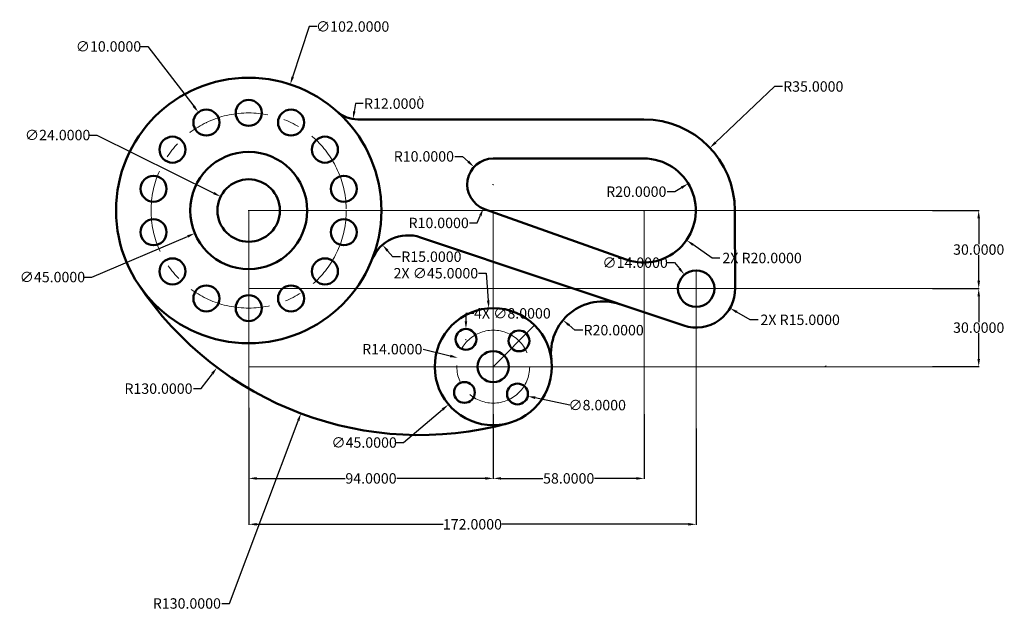
# Model space of a CAD drawing. Units: inches. Extents: x 647 to 1025, y 654 to 881.
import ezdxf

# ---------------------------------------------------------------- set-up
doc = ezdxf.new("R2010")
doc.units = ezdxf.units.IN
doc.header["$MEASUREMENT"] = 0
doc.linetypes.add('CENTER', pattern=[50.8, 31.75, -6.35, 6.35, -6.35])
for name, color, linetype, lineweight in [('M-CNTR', 240, 'CENTER', 18), ('M-CONS', 240, 'Continuous', 13), ('M-DIMS', 2, 'Continuous', 25), ('M-OUTL', 7, 'Continuous', 50)]:
    doc.layers.add(name, color=color, linetype=linetype, lineweight=lineweight)
doc.styles.get("Standard").update_dxf_attribs({"font": 'arial.ttf'})
doc.dimstyles.get("Standard").update_dxf_attribs({"dimtxt": 4, "dimasz": 3, "dimexe": 0.18, "dimexo": 0.0625, "dimgap": 0.09, "dimtad": 0, "dimtih": 1, "dimtoh": 1, "dimdec": 4, "dimzin": 0, "dimdsep": 46, "dimtxsty": 'Standard', "dimcen": 0.09, "dimadec": 0, "dimazin": 0, "dimtfac": 1, "dimtdec": 4, "dimtofl": 0, "dimtmove": 0, "dimatfit": 3, "dimfxl": 1, "dimtolj": 1, "dimtzin": 0, "dimarcsym": 0})

# ---------------------------------------------------------------- blocks, each defined once
blk = doc.blocks.new('*D1')
at = {"layer": 'Defpoints', "color": 0, "transparency": 16777216}
for p in [(750.65, 855.91), (718.74, 759.03)]:
    blk.add_point(p, dxfattribs=at)
at = {"layer": 'M-DIMS', "color": 0, "lineweight": -2, "transparency": 16777216}
for p, q in [((757.98, 878.16), (751.59, 858.76)), ((760.98, 878.16), (757.98, 878.16)), ((734.61, 807.47), (734.79, 807.47)), ((734.7, 807.38), (734.7, 807.56))]:
    blk.add_line(p, q, dxfattribs=at)
at = {"layer": 'M-DIMS', "color": 0, "transparency": 16777216}
blk.add_solid([(751.12, 858.91), (752.07, 858.6), (750.65, 855.91)], dxfattribs=at)
at = {"layer": 'M-DIMS', "color": 0, "transparency": 16777216, "insert": (774.65, 878.16), "char_height": 4, "attachment_point": 5}
blk.add_mtext('\\A1;∅102.0000', dxfattribs=at)
blk = doc.blocks.new('*D2')
at = {"layer": 'Defpoints', "color": 0, "transparency": 16777216}
for p in [(715.38, 845.22), (721.48, 837.29)]:
    blk.add_point(p, dxfattribs=at)
at = {"layer": 'M-DIMS', "color": 0, "lineweight": -2, "transparency": 16777216}
for p, q in [((692.92, 870.5), (695.92, 870.5)), ((695.92, 870.5), (713.55, 847.59)), ((718.34, 841.25), (718.52, 841.25)), ((718.43, 841.16), (718.43, 841.34))]:
    blk.add_line(p, q, dxfattribs=at)
at = {"layer": 'M-DIMS', "color": 0, "transparency": 16777216}
blk.add_solid([(713.94, 847.9), (713.15, 847.29), (715.38, 845.22)], dxfattribs=at)
at = {"layer": 'M-DIMS', "color": 0, "transparency": 16777216, "insert": (680.8, 870.5), "char_height": 4, "attachment_point": 5}
blk.add_mtext('\\A1;∅10.0000', dxfattribs=at)
blk = doc.blocks.new('*D3')
at = {"layer": 'Defpoints', "color": 0, "transparency": 16777216}
for p in [(755.41, 816.25), (713.98, 798.69)]:
    blk.add_point(p, dxfattribs=at)
at = {"layer": 'M-DIMS', "color": 0, "lineweight": -2, "transparency": 16777216}
for p, q in [((734.61, 807.47), (734.79, 807.47)), ((734.7, 807.38), (734.7, 807.56)), ((674.36, 781.9), (711.22, 797.52)), ((671.36, 781.9), (674.36, 781.9))]:
    blk.add_line(p, q, dxfattribs=at)
at = {"layer": 'M-DIMS', "color": 0, "transparency": 16777216}
blk.add_solid([(711.02, 797.98), (711.41, 797.06), (713.98, 798.69)], dxfattribs=at)
at = {"layer": 'M-DIMS', "color": 0, "transparency": 16777216, "insert": (659.25, 781.9), "char_height": 4, "attachment_point": 5}
blk.add_mtext('\\A1;∅45.0000', dxfattribs=at)
blk = doc.blocks.new('*D4')
at = {"layer": 'Defpoints', "color": 0, "transparency": 16777216}
for p in [(723.95, 812.81), (745.44, 802.13)]:
    blk.add_point(p, dxfattribs=at)
at = {"layer": 'M-DIMS', "color": 0, "lineweight": -2, "transparency": 16777216}
for p, q in [((673.37, 836.46), (676.37, 836.46)), ((676.37, 836.46), (721.27, 814.14)), ((734.61, 807.47), (734.79, 807.47)), ((734.7, 807.38), (734.7, 807.56))]:
    blk.add_line(p, q, dxfattribs=at)
at = {"layer": 'M-DIMS', "color": 0, "transparency": 16777216}
blk.add_solid([(721.49, 814.59), (721.04, 813.7), (723.95, 812.81)], dxfattribs=at)
at = {"layer": 'M-DIMS', "color": 0, "transparency": 16777216, "insert": (661.25, 836.46), "char_height": 4, "attachment_point": 5}
blk.add_mtext('\\A1;∅24.0000', dxfattribs=at)
blk = doc.blocks.new('*D5')
at = {"layer": 'Defpoints', "color": 0, "transparency": 16777216}
for p in [(845.89, 761.98), (811.51, 732.95)]:
    blk.add_point(p, dxfattribs=at)
at = {"layer": 'M-DIMS', "color": 0, "lineweight": -2, "transparency": 16777216}
for p, q in [((828.61, 747.47), (828.79, 747.47)), ((828.7, 747.38), (828.7, 747.56)), ((794.18, 718.32), (809.21, 731.02)), ((791.18, 718.32), (794.18, 718.32))]:
    blk.add_line(p, q, dxfattribs=at)
at = {"layer": 'M-DIMS', "color": 0, "transparency": 16777216}
blk.add_solid([(808.89, 731.4), (809.54, 730.63), (811.51, 732.95)], dxfattribs=at)
at = {"layer": 'M-DIMS', "color": 0, "transparency": 16777216, "insert": (779.06, 718.32), "char_height": 4, "attachment_point": 5}
blk.add_mtext('\\A1;∅45.0000', dxfattribs=at)
blk = doc.blocks.new('*D6')
at = {"layer": 'Defpoints', "color": 0, "transparency": 16777216}
for p in [(834.1, 737.82), (841.92, 736.15)]:
    blk.add_point(p, dxfattribs=at)
at = {"layer": 'M-DIMS', "color": 0, "lineweight": -2, "transparency": 16777216}
for p, q in [((837.92, 736.98), (838.1, 736.98)), ((838.01, 736.89), (838.01, 737.07)), ((858.09, 732.7), (844.86, 735.52))]:
    blk.add_line(p, q, dxfattribs=at)
at = {"layer": 'M-DIMS', "color": 0, "transparency": 16777216}
blk.add_solid([(844.96, 736.01), (844.75, 735.03), (841.92, 736.15)], dxfattribs=at)
at = {"layer": 'M-DIMS', "color": 0, "transparency": 16777216, "insert": (868.65, 732.7), "char_height": 4, "attachment_point": 5}
blk.add_mtext('\\A1;∅8.0000', dxfattribs=at)
blk = doc.blocks.new('*D7')
at = {"layer": 'Defpoints', "color": 0, "transparency": 16777216}
for p in [(800.49, 851.2), (722.53, 747.17)]:
    blk.add_point(p, dxfattribs=at)
at = {"layer": 'M-DIMS', "color": 0, "lineweight": -2, "transparency": 16777216}
for p, q in [((800.4, 851.2), (800.58, 851.2)), ((800.49, 851.11), (800.49, 851.29)), ((716.43, 739.03), (720.73, 744.77)), ((713.43, 739.03), (716.43, 739.03))]:
    blk.add_line(p, q, dxfattribs=at)
at = {"layer": 'M-DIMS', "color": 0, "transparency": 16777216}
blk.add_solid([(720.33, 745.07), (721.13, 744.47), (722.53, 747.17)], dxfattribs=at)
at = {"layer": 'M-DIMS', "color": 0, "transparency": 16777216, "insert": (700.02, 739.03), "char_height": 4, "attachment_point": 5}
blk.add_mtext('\\A1;R130.0000', dxfattribs=at)
blk = doc.blocks.new('*D8')
at = {"layer": 'Defpoints', "color": 0, "transparency": 16777216}
for p in [(911.96, 831.54), (886.56, 807.47)]:
    blk.add_point(p, dxfattribs=at)
at = {"layer": 'M-DIMS', "color": 0, "lineweight": -2, "transparency": 16777216}
for p, q in [((936.85, 855.12), (914.14, 833.6)), ((939.85, 855.12), (936.85, 855.12)), ((886.47, 807.47), (886.65, 807.47)), ((886.56, 807.38), (886.56, 807.56))]:
    blk.add_line(p, q, dxfattribs=at)
at = {"layer": 'M-DIMS', "color": 0, "transparency": 16777216}
blk.add_solid([(913.8, 833.97), (914.49, 833.24), (911.96, 831.54)], dxfattribs=at)
at = {"layer": 'M-DIMS', "color": 0, "transparency": 16777216, "insert": (951.71, 855.12), "char_height": 4, "attachment_point": 5}
blk.add_mtext('\\A1;R35.0000', dxfattribs=at)
blk = doc.blocks.new('*D9')
at = {"layer": 'Defpoints', "color": 0, "transparency": 16777216}
for p in [(903.67, 817.82), (886.56, 807.47)]:
    blk.add_point(p, dxfattribs=at)
at = {"layer": 'M-DIMS', "color": 0, "lineweight": -2, "transparency": 16777216}
for p, q in [((895.54, 814.71), (898.54, 814.71)), ((898.54, 814.71), (901.1, 816.27))]:
    blk.add_line(p, q, dxfattribs=at)
at = {"layer": 'M-DIMS', "color": 0, "transparency": 16777216}
blk.add_solid([(900.84, 816.69), (901.36, 815.84), (903.67, 817.82)], dxfattribs=at)
at = {"layer": 'M-DIMS', "color": 0, "transparency": 16777216, "insert": (883.68, 814.71), "char_height": 4, "attachment_point": 5}
blk.add_mtext('\\A1;R20.0000', dxfattribs=at)
blk = doc.blocks.new('*D10')
at = {"layer": 'Defpoints', "color": 0, "transparency": 16777216}
for p in [(821.31, 824.21), (828.7, 817.47)]:
    blk.add_point(p, dxfattribs=at)
at = {"layer": 'M-DIMS', "color": 0, "lineweight": -2, "transparency": 16777216}
for p, q in [((813.88, 828.26), (816.88, 828.26)), ((816.88, 828.26), (819.1, 826.24)), ((828.7, 817.38), (828.7, 817.56)), ((828.61, 817.47), (828.79, 817.47))]:
    blk.add_line(p, q, dxfattribs=at)
at = {"layer": 'M-DIMS', "color": 0, "transparency": 16777216}
blk.add_solid([(819.44, 826.61), (818.76, 825.87), (821.31, 824.21)], dxfattribs=at)
at = {"layer": 'M-DIMS', "color": 0, "transparency": 16777216, "insert": (802.03, 828.26), "char_height": 4, "attachment_point": 5}
blk.add_mtext('\\A1;R10.0000', dxfattribs=at)
blk = doc.blocks.new('*D11')
at = {"layer": 'Defpoints', "color": 0, "transparency": 16777216}
for p in [(786.13, 794.26), (795.97, 782.93)]:
    blk.add_point(p, dxfattribs=at)
at = {"layer": 'M-DIMS', "color": 0, "lineweight": -2, "transparency": 16777216}
for p, q in [((790.07, 789.73), (788.1, 791.99)), ((793.07, 789.73), (790.07, 789.73))]:
    blk.add_line(p, q, dxfattribs=at)
at = {"layer": 'M-DIMS', "color": 0, "transparency": 16777216}
blk.add_solid([(788.48, 792.32), (787.72, 791.66), (786.13, 794.26)], dxfattribs=at)
at = {"layer": 'M-DIMS', "color": 0, "transparency": 16777216, "insert": (804.92, 789.73), "char_height": 4, "attachment_point": 5}
blk.add_mtext('\\A1;R15.0000', dxfattribs=at)
blk = doc.blocks.new('*D12')
at = {"layer": 'Defpoints', "color": 0, "transparency": 16777216}
for p in [(855.51, 765.34), (870.89, 752.55)]:
    blk.add_point(p, dxfattribs=at)
at = {"layer": 'M-DIMS', "color": 0, "lineweight": -2, "transparency": 16777216}
for p, q in [((860.12, 761.5), (857.82, 763.42)), ((863.12, 761.5), (860.12, 761.5))]:
    blk.add_line(p, q, dxfattribs=at)
at = {"layer": 'M-DIMS', "color": 0, "transparency": 16777216}
blk.add_solid([(858.14, 763.8), (857.5, 763.03), (855.51, 765.34)], dxfattribs=at)
at = {"layer": 'M-DIMS', "color": 0, "transparency": 16777216, "insert": (874.98, 761.5), "char_height": 4, "attachment_point": 5}
blk.add_mtext('\\A1;R20.0000', dxfattribs=at)
blk = doc.blocks.new('*D13')
at = {"layer": 'Defpoints', "color": 0, "transparency": 16777216}
for p in [(815.11, 750.86), (828.7, 747.47)]:
    blk.add_point(p, dxfattribs=at)
at = {"layer": 'M-DIMS', "color": 0, "lineweight": -2, "transparency": 16777216}
for p, q in [((801.75, 754.2), (812.2, 751.59)), ((828.61, 747.47), (828.79, 747.47)), ((828.7, 747.38), (828.7, 747.56))]:
    blk.add_line(p, q, dxfattribs=at)
at = {"layer": 'M-DIMS', "color": 0, "transparency": 16777216}
blk.add_solid([(812.33, 752.07), (812.08, 751.1), (815.11, 750.86)], dxfattribs=at)
at = {"layer": 'M-DIMS', "color": 0, "transparency": 16777216, "insert": (789.89, 754.2), "char_height": 4, "attachment_point": 5}
blk.add_mtext('\\A1;R14.0000', dxfattribs=at)
blk = doc.blocks.new('*D14')
at = {"layer": 'Defpoints', "color": 0, "transparency": 16777216}
for p in [(776.65, 854.47), (774.82, 842.61)]:
    blk.add_point(p, dxfattribs=at)
at = {"layer": 'M-DIMS', "color": 0, "lineweight": -2, "transparency": 16777216}
for p, q in [((775.73, 848.54), (775.27, 845.57)), ((778.73, 848.54), (775.73, 848.54))]:
    blk.add_line(p, q, dxfattribs=at)
at = {"layer": 'M-DIMS', "color": 0, "transparency": 16777216}
blk.add_solid([(774.78, 845.65), (775.77, 845.5), (774.82, 842.61)], dxfattribs=at)
at = {"layer": 'M-DIMS', "color": 0, "transparency": 16777216, "insert": (790.59, 848.54), "char_height": 4, "attachment_point": 5}
blk.add_mtext('\\A1;R12.0000', dxfattribs=at)
blk = doc.blocks.new('*D15')
at = {"layer": 'Defpoints', "color": 0, "transparency": 16777216}
for p in [(734.7, 723.79), (906.7, 723.79), (906.7, 686.9)]:
    blk.add_point(p, dxfattribs=at)
at = {"layer": 'M-DIMS', "color": 0, "lineweight": -2, "transparency": 16777216}
for p, q in [((734.7, 723.73), (734.7, 686.72)), ((906.7, 723.73), (906.7, 686.72)), ((737.7, 686.9), (809.39, 686.9)), ((903.7, 686.9), (832, 686.9))]:
    blk.add_line(p, q, dxfattribs=at)
at = {"layer": 'M-DIMS', "color": 0, "transparency": 16777216}
for points in [[(737.7, 687.4), (737.7, 686.4), (734.7, 686.9)], [(903.7, 687.4), (903.7, 686.4), (906.7, 686.9)]]:
    blk.add_solid(points, dxfattribs=at)
at = {"layer": 'M-DIMS', "color": 0, "transparency": 16777216, "insert": (820.7, 686.9), "char_height": 4, "attachment_point": 5}
blk.add_mtext('\\A1;172.0000', dxfattribs=at)
blk = doc.blocks.new('*D16')
at = {"layer": 'Defpoints', "color": 0, "transparency": 16777216}
for p in [(734.7, 731.75), (828.7, 729.23), (828.7, 704.54)]:
    blk.add_point(p, dxfattribs=at)
at = {"layer": 'M-DIMS', "color": 0, "lineweight": -2, "transparency": 16777216}
for p, q in [((734.7, 731.69), (734.7, 704.36)), ((828.7, 729.17), (828.7, 704.36)), ((737.7, 704.54), (771.76, 704.54)), ((825.7, 704.54), (791.64, 704.54))]:
    blk.add_line(p, q, dxfattribs=at)
at = {"layer": 'M-DIMS', "color": 0, "transparency": 16777216}
for points in [[(737.7, 705.04), (737.7, 704.04), (734.7, 704.54)], [(825.7, 705.04), (825.7, 704.04), (828.7, 704.54)]]:
    blk.add_solid(points, dxfattribs=at)
at = {"layer": 'M-DIMS', "color": 0, "transparency": 16777216, "insert": (781.7, 704.54), "char_height": 4, "attachment_point": 5}
blk.add_mtext('\\A1;94.0000', dxfattribs=at)
blk = doc.blocks.new('*D17')
at = {"layer": 'Defpoints', "color": 0, "transparency": 16777216}
for p in [(828.7, 729.23), (886.7, 729.23), (886.7, 704.54)]:
    blk.add_point(p, dxfattribs=at)
at = {"layer": 'M-DIMS', "color": 0, "lineweight": -2, "transparency": 16777216}
for p, q in [((828.7, 729.17), (828.7, 704.36)), ((886.7, 729.17), (886.7, 704.36)), ((831.7, 704.54), (847.76, 704.54)), ((883.7, 704.54), (867.64, 704.54))]:
    blk.add_line(p, q, dxfattribs=at)
at = {"layer": 'M-DIMS', "color": 0, "transparency": 16777216}
for points in [[(831.7, 705.04), (831.7, 704.04), (828.7, 704.54)], [(883.7, 705.04), (883.7, 704.04), (886.7, 704.54)]]:
    blk.add_solid(points, dxfattribs=at)
at = {"layer": 'M-DIMS', "color": 0, "transparency": 16777216, "insert": (857.7, 704.54), "char_height": 4, "attachment_point": 5}
blk.add_mtext('\\A1;58.0000', dxfattribs=at)
blk = doc.blocks.new('HOLE-D10')
blk.add_circle((5, 5), 5)
blk = doc.blocks.new('HOLE-D8')
blk.add_circle((4, 4), 4)
blk = doc.blocks.new('*D20')
at = {"layer": 'Defpoints', "color": 0, "transparency": 16777216}
for p in [(997.45, 807.47), (997.45, 777.47), (1015.3, 777.47)]:
    blk.add_point(p, dxfattribs=at)
at = {"layer": 'M-DIMS', "color": 0, "lineweight": -2, "transparency": 16777216}
for p, q in [((997.51, 807.47), (1015.48, 807.47)), ((1015.3, 804.47), (1015.3, 794.6)), ((1015.3, 780.47), (1015.3, 790.33)), ((997.51, 777.47), (1015.48, 777.47))]:
    blk.add_line(p, q, dxfattribs=at)
at = {"layer": 'M-DIMS', "color": 0, "transparency": 16777216}
for points in [[(1014.8, 804.47), (1015.8, 804.47), (1015.3, 807.47)], [(1014.8, 780.47), (1015.8, 780.47), (1015.3, 777.47)]]:
    blk.add_solid(points, dxfattribs=at)
at = {"layer": 'M-DIMS', "color": 0, "transparency": 16777216, "insert": (1015.3, 792.47), "char_height": 4, "attachment_point": 5}
blk.add_mtext('\\A1;30.0000', dxfattribs=at)
blk = doc.blocks.new('*D21')
at = {"layer": 'Defpoints', "color": 0, "transparency": 16777216}
for p in [(997.45, 777.47), (997.45, 747.47), (1015.3, 747.47)]:
    blk.add_point(p, dxfattribs=at)
at = {"layer": 'M-DIMS', "color": 0, "lineweight": -2, "transparency": 16777216}
for p, q in [((997.51, 777.47), (1015.48, 777.47)), ((1015.3, 774.47), (1015.3, 764.6)), ((1015.3, 750.47), (1015.3, 760.33)), ((997.51, 747.47), (1015.48, 747.47))]:
    blk.add_line(p, q, dxfattribs=at)
at = {"layer": 'M-DIMS', "color": 0, "transparency": 16777216}
for points in [[(1014.8, 774.47), (1015.8, 774.47), (1015.3, 777.47)], [(1014.8, 750.47), (1015.8, 750.47), (1015.3, 747.47)]]:
    blk.add_solid(points, dxfattribs=at)
at = {"layer": 'M-DIMS', "color": 0, "transparency": 16777216, "insert": (1015.3, 762.47), "char_height": 4, "attachment_point": 5}
blk.add_mtext('\\A1;30.0000', dxfattribs=at)
blk = doc.blocks.new('*D22')
at = {"layer": 'Defpoints', "color": 0, "transparency": 16777216}
for p in [(827, 769.9), (830.39, 725.03)]:
    blk.add_point(p, dxfattribs=at)
at = {"layer": 'M-DIMS', "color": 0, "lineweight": -2, "transparency": 16777216}
for p, q in [((822.98, 783.37), (825.98, 783.37)), ((825.98, 783.37), (826.77, 772.9)), ((828.61, 747.47), (828.79, 747.47)), ((828.7, 747.38), (828.7, 747.56))]:
    blk.add_line(p, q, dxfattribs=at)
at = {"layer": 'M-DIMS', "color": 0, "transparency": 16777216}
blk.add_solid([(827.27, 772.93), (826.27, 772.86), (827, 769.9)], dxfattribs=at)
at = {"layer": 'M-DIMS', "color": 0, "transparency": 16777216, "insert": (806.64, 783.37), "char_height": 4, "attachment_point": 5}
blk.add_mtext('\\A1;2X ∅45.0000', dxfattribs=at)
blk = doc.blocks.new('*D23')
at = {"layer": 'Defpoints', "color": 0, "transparency": 16777216}
for p in [(828.7, 817.47), (824.87, 808.23)]:
    blk.add_point(p, dxfattribs=at)
at = {"layer": 'M-DIMS', "color": 0, "lineweight": -2, "transparency": 16777216}
for p, q in [((828.7, 817.38), (828.7, 817.56)), ((828.61, 817.47), (828.79, 817.47)), ((819.57, 802.69), (822.57, 802.69)), ((822.57, 802.69), (823.72, 805.46))]:
    blk.add_line(p, q, dxfattribs=at)
at = {"layer": 'M-DIMS', "color": 0, "transparency": 16777216}
blk.add_solid([(823.26, 805.65), (824.18, 805.27), (824.87, 808.23)], dxfattribs=at)
at = {"layer": 'M-DIMS', "color": 0, "transparency": 16777216, "insert": (807.72, 802.69), "char_height": 4, "attachment_point": 5}
blk.add_mtext('\\A1;R10.0000', dxfattribs=at)
blk = doc.blocks.new('*D24')
at = {"layer": 'Defpoints', "color": 0, "transparency": 16777216}
for p in [(886.56, 807.47), (902.98, 796.06)]:
    blk.add_point(p, dxfattribs=at)
at = {"layer": 'M-DIMS', "color": 0, "lineweight": -2, "transparency": 16777216}
for p, q in [((886.47, 807.47), (886.65, 807.47)), ((886.56, 807.38), (886.56, 807.56)), ((912.84, 789.22), (905.45, 794.35)), ((915.84, 789.22), (912.84, 789.22))]:
    blk.add_line(p, q, dxfattribs=at)
at = {"layer": 'M-DIMS', "color": 0, "transparency": 16777216}
blk.add_solid([(905.73, 794.76), (905.16, 793.94), (902.98, 796.06)], dxfattribs=at)
at = {"layer": 'M-DIMS', "color": 0, "transparency": 16777216, "insert": (932.03, 789.22), "char_height": 4, "attachment_point": 5}
blk.add_mtext('\\A1;2X R20.0000', dxfattribs=at)
blk = doc.blocks.new('*D25')
at = {"layer": 'Defpoints', "color": 0, "transparency": 16777216}
for p in [(906.7, 777.47), (919.69, 769.97)]:
    blk.add_point(p, dxfattribs=at)
at = {"layer": 'M-DIMS', "color": 0, "lineweight": -2, "transparency": 16777216}
for p, q in [((906.61, 777.47), (906.79, 777.47)), ((906.7, 777.38), (906.7, 777.56)), ((927.48, 765.47), (922.29, 768.47)), ((930.48, 765.47), (927.48, 765.47))]:
    blk.add_line(p, q, dxfattribs=at)
at = {"layer": 'M-DIMS', "color": 0, "transparency": 16777216}
blk.add_solid([(922.54, 768.9), (922.04, 768.04), (919.69, 769.97)], dxfattribs=at)
at = {"layer": 'M-DIMS', "color": 0, "transparency": 16777216, "insert": (946.67, 765.47), "char_height": 4, "attachment_point": 5}
blk.add_mtext('\\A1;2X R15.0000', dxfattribs=at)
blk = doc.blocks.new('*D26')
at = {"layer": 'Defpoints', "color": 0, "transparency": 16777216}
for p in [(902.2, 782.83), (911.2, 772.1)]:
    blk.add_point(p, dxfattribs=at)
at = {"layer": 'M-DIMS', "color": 0, "lineweight": -2, "transparency": 16777216}
for p, q in [((895.34, 787.43), (898.34, 787.43)), ((898.34, 787.43), (900.27, 785.13)), ((906.61, 777.47), (906.79, 777.47)), ((906.7, 777.38), (906.7, 777.56))]:
    blk.add_line(p, q, dxfattribs=at)
at = {"layer": 'M-DIMS', "color": 0, "transparency": 16777216}
blk.add_solid([(900.65, 785.45), (899.89, 784.81), (902.2, 782.83)], dxfattribs=at)
at = {"layer": 'M-DIMS', "color": 0, "transparency": 16777216, "insert": (883.23, 787.43), "char_height": 4, "attachment_point": 5}
blk.add_mtext('\\A1;∅14.0000', dxfattribs=at)
blk = doc.blocks.new('*D27')
at = {"layer": 'Defpoints', "color": 0, "transparency": 16777216}
for p in [(800.49, 851.2), (754.78, 729.5)]:
    blk.add_point(p, dxfattribs=at)
at = {"layer": 'M-DIMS', "color": 0, "lineweight": -2, "transparency": 16777216}
for p, q in [((800.4, 851.2), (800.58, 851.2)), ((800.49, 851.11), (800.49, 851.29)), ((727.35, 656.48), (753.72, 726.69)), ((724.35, 656.48), (727.35, 656.48))]:
    blk.add_line(p, q, dxfattribs=at)
at = {"layer": 'M-DIMS', "color": 0, "transparency": 16777216}
blk.add_solid([(753.25, 726.87), (754.19, 726.52), (754.78, 729.5)], dxfattribs=at)
at = {"layer": 'M-DIMS', "color": 0, "transparency": 16777216, "insert": (710.94, 656.48), "char_height": 4, "attachment_point": 5}
blk.add_mtext('\\A1;R130.0000', dxfattribs=at)
blk = doc.blocks.new('*D28')
at = {"layer": 'Defpoints', "color": 0, "transparency": 16777216}
for p in [(818.21, 761.95), (818.21, 753.95)]:
    blk.add_point(p, dxfattribs=at)
at = {"layer": 'M-DIMS', "color": 0, "lineweight": -2, "transparency": 16777216}
for p, q in [((821.21, 767.95), (818.21, 767.95)), ((818.21, 767.95), (818.21, 764.95)), ((818.12, 757.95), (818.3, 757.95)), ((818.21, 757.86), (818.21, 758.04))]:
    blk.add_line(p, q, dxfattribs=at)
at = {"layer": 'M-DIMS', "color": 0, "transparency": 16777216}
blk.add_solid([(817.71, 764.95), (818.71, 764.95), (818.21, 761.95)], dxfattribs=at)
at = {"layer": 'M-DIMS', "color": 0, "transparency": 16777216, "insert": (836.05, 767.95), "char_height": 4, "attachment_point": 5}
blk.add_mtext('\\A1;4X ∅8.0000', dxfattribs=at)

msp = doc.modelspace()

# ---------------------------------------------------------------- linework, layer by layer
at = {"layer": 'M-CNTR'}
for centre, radius in [((734.69735, 807.46805), 37.5), ((828.69735, 747.46805), 14)]:
    msp.add_circle(centre, radius, dxfattribs=at)
at = {"layer": 'M-CONS'}
for p, q in [((734.69735, 807.46805), (734.69735, 723.7887)), ((734.69735, 807.46805), (997.44528, 807.46805)), ((828.69735, 807.46805), (828.69735, 723.7887)), ((886.69735, 807.46805), (886.69735, 723.7887)), ((906.69735, 784.46805), (906.69735, 723.7887)), ((734.69735, 777.46805), (997.44528, 777.46805)), ((858.69735, 777.46805), (858.89493, 777.66563)), ((828.69735, 747.46805), (844.60725, 763.37795)), ((734.69735, 747.46805), (997.44528, 747.46805))]:
    msp.add_line(p, q, dxfattribs=at)
msp.add_arc((848.04451, 987.3802), 263.1244, 294.2471844, 294.3871536, dxfattribs=at)
at = {"layer": 'M-OUTL'}
for p, q in [((886.5562, 842.46805), (776.6497, 842.46805)), ((886.5562, 827.46805), (828.69735, 827.46805)), ((879.84335, 788.62826), (825.34093, 808.04816)), ((921.5562, 807.46805), (921.69735, 777.46805)), ((901.93169, 763.24524), (800.73252, 797.15421))]:
    msp.add_line(p, q, dxfattribs=at)
for centre, radius in [((734.69735, 807.46805), 51), ((734.69735, 807.46805), 22.5), ((734.69735, 807.46805), 12), ((906.69735, 777.46805), 7), ((828.69735, 747.46805), 22.5), ((828.69735, 747.46805), 6)]:
    msp.add_circle(centre, radius, dxfattribs=at)
for centre, radius, start, end in [((776.6497, 854.46805), 12, 228.2477948, 270), ((886.5562, 807.46805), 35, 0, 90), ((828.69735, 817.46805), 10, 90, 250.3883825), ((886.5562, 807.46805), 20, 250.3883825, 90), ((795.96686, 782.9314), 15, 71.4754578, 158.1753358), ((800.48824, 851.20086), 130, 213.6129566, 285.2131305), ((906.69735, 777.46805), 15, 251.4754578, 0.5391431), ((870.89207, 752.55286), 20, 71.4754578, 186.8714754)]:
    msp.add_arc(centre, radius, start, end, dxfattribs=at)

# ---------------------------------------------------------------- block references
for name, p in [('HOLE-D10', (729.697, 839.968)), ('HOLE-D10', (713.42636, 836.25433)), ('HOLE-D10', (745.96764, 836.25433)), ('HOLE-D10', (700.37832, 825.84887)), ('HOLE-D10', (759.01568, 825.84887)), ('HOLE-D10', (693.1372, 810.81254)), ('HOLE-D10', (766.2568, 810.81254)), ('HOLE-D10', (693.1372, 794.12346)), ('HOLE-D10', (766.2568, 794.12346)), ('HOLE-D10', (700.37832, 779.08713)), ('HOLE-D10', (759.01568, 779.08713)), ('HOLE-D10', (713.42636, 768.68167)), ('HOLE-D10', (745.96764, 768.68167)), ('HOLE-D10', (729.697, 764.968)), ('HOLE-D8', (814.21283, 753.95318)), ('HOLE-D8', (834.597, 753.368)), ('HOLE-D8', (813.62764, 733.56901)), ('HOLE-D8', (834.01182, 732.98383))]:
    msp.add_blockref(name, p, dxfattribs=at)

# ---------------------------------------------------------------- dimensions: what is measured, and where the dimension line sits
at = {"layer": 'M-DIMS'}
for p1, p2, override, picture, middle in [((718.74008, 759.02876), (750.65463, 855.90735), {"dimclrd": 0, "dimclre": 0, "dimclrt": 0}, '*D1', (774.65449, 878.15819)), ((721.4762, 837.29198), (715.37722, 845.21679), {"dimclrd": 0, "dimclre": 0, "dimclrt": 0}, '*D2', (680.80291, 870.50037)), ((745.44318, 802.12696), (723.95153, 812.80914), {"dimclrd": 0, "dimclre": 0, "dimclrt": 0}, '*D4', (661.25113, 836.46046)), ((755.41357, 816.24805), (713.98113, 798.68805), {"dimclrd": 0, "dimclre": 0, "dimclrt": 0}, '*D3', (659.24582, 781.89647)), ((911.19577, 772.10482), (902.19893, 782.83128), {"dimdec": 4, "dimlfac": 1, "dimrnd": 0, "dimzin": 0, "dimdsep": 46, "dimlunit": 2}, '*D26', (883.22722, 787.42833)), ((845.88867, 761.98386), (811.50603, 732.95225), {"dimclrd": 0, "dimclre": 0, "dimclrt": 0}, '*D5', (779.06316, 718.32192)), ((834.09971, 737.81802), (841.92361, 736.14872), {"dimclrd": 0, "dimclre": 0, "dimclrt": 0}, '*D6', (858.09174, 732.69911))]:
    dim = msp.add_diameter_dim_2p(p1=p1, p2=p2, dimstyle='Standard', override=override, dxfattribs=at)
    dim.commit()
    dim.dimension.update_dxf_attribs({"geometry": picture, "text_midpoint": middle, "dimtype": 163})
for center, mpoint, override, picture, middle in [((886.5562, 807.46805), (911.96434, 831.53933), {"dimclrd": 0, "dimclre": 0, "dimclrt": 0}, '*D8', (951.70855, 855.11996)), ((776.6497, 854.46805), (774.81555, 842.60905), {"dimclrd": 0, "dimclre": 0, "dimclrt": 0}, '*D14', (790.58661, 848.53855)), ((800.48824, 851.20086), (722.52654, 747.17215), {"dimclrd": 0, "dimclre": 0, "dimclrt": 0}, '*D7', (700.01725, 739.03069)), ((800.48824, 851.20086), (754.77685, 729.50259), {"dimdec": 4, "dimlfac": 1, "dimrnd": 0, "dimzin": 0, "dimdsep": 46, "dimlunit": 2}, '*D27', (710.94214, 656.48363)), ((828.69735, 817.46805), (824.86725, 808.23061), {"dimdec": 4, "dimlfac": 1, "dimrnd": 0, "dimzin": 0, "dimdsep": 46, "dimlunit": 2}, '*D23', (807.71521, 802.68814)), ((886.5562, 807.46805), (903.66963, 817.81844), {"dimclrd": 0, "dimclre": 0, "dimclrt": 0}, '*D9', (883.68162, 814.71333)), ((795.96686, 782.9314), (786.13195, 794.25723), {"dimclrd": 0, "dimclre": 0, "dimclrt": 0}, '*D11', (804.9199, 789.7269)), ((870.89207, 752.55286), (855.51049, 765.33593), {"dimclrd": 0, "dimclre": 0, "dimclrt": 0}, '*D12', (874.97895, 761.50101)), ((828.69735, 747.46805), (815.11449, 750.86009), {"dimclrd": 0, "dimclre": 0, "dimclrt": 0}, '*D13', (801.74731, 754.19827))]:
    dim = msp.add_radius_dim(center=center, mpoint=mpoint, dimstyle='Standard', override=override, dxfattribs=at)
    dim.commit()
    dim.dimension.update_dxf_attribs({"geometry": picture, "text_midpoint": middle, "dimtype": 164})
dim = msp.add_radius_dim(center=(828.69735, 817.46805), mpoint=(821.31462, 824.21307), dimstyle='Standard', override={"dimclrd": 0, "dimclre": 0, "dimclrt": 0}, dxfattribs=at)
dim.commit()
dim.dimension.update_dxf_attribs({"geometry": '*D10', "text_midpoint": (802.031, 828.26009)})
for center, mpoint, picture, middle in [((886.5562, 807.46805), (902.98444, 796.06135), '*D24', (932.02689, 789.21733)), ((906.69735, 777.46805), (919.68828, 769.96899), '*D25', (946.66833, 765.46956))]:
    dim = msp.add_radius_dim(center=center, mpoint=mpoint, text='2X <>', dimstyle='Standard', override={"dimdec": 4, "dimlfac": 1, "dimrnd": 0, "dimzin": 0, "dimdsep": 46, "dimlunit": 2}, dxfattribs=at)
    dim.commit()
    dim.dimension.update_dxf_attribs({"geometry": picture, "text_midpoint": middle, "dimtype": 164})
for base, p1, p2, picture, middle in [((1015.29528, 777.46805), (997.44528, 807.46805), (997.44528, 777.46805), '*D20', (1015.29528, 792.46805)), ((1015.29528, 747.46805), (997.44528, 777.46805), (997.44528, 747.46805), '*D21', (1015.29528, 762.46805))]:
    dim = msp.add_linear_dim(base=base, p1=p1, p2=p2, angle=90, dimstyle='Standard', override={"dimdec": 4, "dimlfac": 1, "dimrnd": 0, "dimzin": 0, "dimdsep": 46, "dimlunit": 2}, dxfattribs=at)
    dim.commit()
    dim.dimension.update_dxf_attribs({"geometry": picture, "text_midpoint": middle})
for p1, p2, text, picture, middle in [((830.395, 725.03219), (826.9997, 769.90391), '2X <>', '*D22', (806.64009, 783.36543)), ((818.21235, 753.95273), (818.213, 761.95273), '4X <>', '*D28', (836.04701, 767.95273))]:
    dim = msp.add_diameter_dim_2p(p1=p1, p2=p2, text=text, dimstyle='Standard', override={"dimdec": 4, "dimlfac": 1, "dimrnd": 0, "dimzin": 0, "dimdsep": 46, "dimlunit": 2}, dxfattribs=at)
    dim.commit()
    dim.dimension.update_dxf_attribs({"geometry": picture, "text_midpoint": middle, "dimtype": 163})
for base, p1, p2, picture, middle in [((828.69735, 704.53711), (734.69735, 731.7499), (828.69735, 729.2302), '*D16', (781.69735, 704.53711)), ((886.69735, 704.53711), (828.69735, 729.2302), (886.69735, 729.2302), '*D17', (857.69735, 704.53711)), ((906.69735, 686.89919), (734.69735, 723.7887), (906.69735, 723.7887), '*D15', (820.69735, 686.89919))]:
    dim = msp.add_linear_dim(base=base, p1=p1, p2=p2, dimstyle='Standard', override={"dimclrd": 0, "dimclre": 0, "dimclrt": 0}, dxfattribs=at)
    dim.commit()
    dim.dimension.update_dxf_attribs({"geometry": picture, "text_midpoint": middle})

doc.saveas('drawing.dxf')
